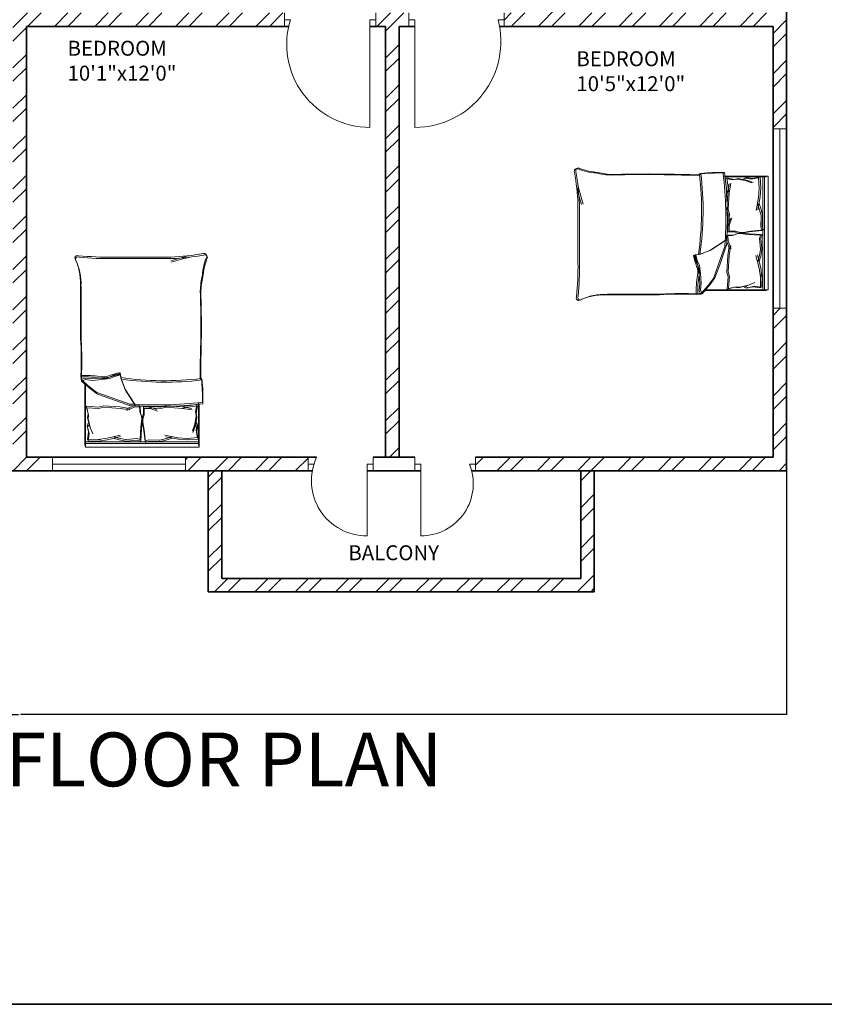
# Model space of a CAD drawing. Units: inches. Extents: x 1944 to 3454, y 1352 to 3055.
# Tile 3 of 17: x 2314 to 2582, y 1352 to 1681. Entities that reach past the tile are written whole.
import ezdxf

# ---------------------------------------------------------------- set-up
doc = ezdxf.new("R2010")
doc.units = ezdxf.units.IN
for name, color, linetype, lineweight in [('A-ANNO-DIMS', 2, 'Continuous', 18), ('A-ANNO-TITL', 7, 'Continuous', 30), ('A-ANNO-TTLB', 7, 'Continuous', 35), ('A-AREA-IDEN', 7, 'Continuous', 18), ('A-DOOR', 3, 'Continuous', 20), ('A-FURN', 8, 'Continuous', 13), ('A-GLAZ', 4, 'Continuous', 18), ('A-WALL', 7, 'Continuous', 35), ('A-WALL-PATT', 252, 'Continuous', 13)]:
    doc.layers.add(name, color=color, linetype=linetype, lineweight=lineweight)
doc.styles.get("Standard").update_dxf_attribs({"font": 'arial.ttf'})
doc.dimstyles.get("Standard").update_dxf_attribs({"dimtxt": 0.18, "dimasz": 0.18, "dimexe": 0.18, "dimexo": 0.0625, "dimgap": 0.09, "dimtad": 0, "dimtih": 1, "dimtoh": 1, "dimdec": 4, "dimzin": 0, "dimdsep": 46, "dimtxsty": 'Standard', "dimcen": 0.09, "dimadec": 0, "dimazin": 0, "dimtfac": 1, "dimtdec": 4, "dimtofl": 0, "dimtmove": 0, "dimatfit": 3, "dimfxl": 1, "dimtolj": 1, "dimtzin": 0, "dimarcsym": 0})

# ---------------------------------------------------------------- blocks, each defined once
blk = doc.blocks.new('BED-WITH-PILLOWS-01')
for p, q in [((0, 40.75), (21.15, 40.75)), ((0, 40.75), (21.15, 40.75)), ((0, 2.76), (0, 40.75)), ((0.51, 40.93), (21.66, 40.93)), ((0.51, 40.93), (21.66, 40.93)), ((1.22, 2.76), (1.22, 40.75)), ((1.22, 2.76), (1.22, 40.75)), ((1.73, 2.94), (1.73, 40.93)), ((1.73, 2.94), (1.73, 40.93)), ((2.03, 39.83), (1.96, 35.54)), ((2.03, 39.83), (1.96, 35.54)), ((2.03, 39.83), (4.58, 39.53)), ((2.03, 39.83), (4.58, 39.53)), ((2.54, 40.01), (2.46, 35.72)), ((2.54, 40.01), (2.46, 35.72)), ((2.54, 40.01), (5.09, 39.71)), ((2.54, 40.01), (5.09, 39.71)), ((4.58, 39.53), (6.63, 40.01)), ((4.58, 39.53), (6.63, 40.01)), ((5.09, 39.71), (7.14, 40.19)), ((5.09, 39.71), (7.14, 40.19)), ((9.4, 39.83), (6.56, 39.2)), ((9.4, 39.83), (6.56, 39.2)), ((6.63, 40.01), (7.46, 39.6)), ((6.63, 40.01), (7.46, 39.6)), ((9.91, 40.01), (7.07, 39.38)), ((9.91, 40.01), (7.07, 39.38)), ((7.14, 40.19), (7.97, 39.78)), ((7.14, 40.19), (7.97, 39.78)), ((10.68, 39.68), (9.4, 39.83)), ((10.68, 39.68), (9.4, 39.83)), ((11.19, 39.86), (9.91, 40.01)), ((11.19, 39.86), (9.91, 40.01)), ((13.17, 40.3), (10.68, 39.68)), ((13.17, 40.3), (10.68, 39.68)), ((13.68, 40.48), (11.19, 39.86)), ((13.68, 40.48), (11.19, 39.86)), ((12.85, 36.22), (13.17, 40.3)), ((12.85, 36.22), (13.17, 40.3)), ((13.36, 36.4), (13.68, 40.48)), ((13.36, 36.4), (13.68, 40.48)), ((22.05, 42.02), (19.47, 39.08)), ((22.05, 42.02), (19.47, 39.08)), ((22.56, 42.21), (19.98, 39.26)), ((22.56, 42.21), (19.98, 39.26)), ((23.44, 42.09), (22.05, 42.02, 3.08)), ((23.44, 42.09), (22.05, 42.02, 3.08)), ((22.55, 40.8), (22.05, 42.02)), ((22.55, 40.8), (22.05, 42.02)), ((22.3, 38.34), (22.55, 40.8)), ((22.3, 38.34), (22.55, 40.8)), ((23.95, 42.27), (22.56, 42.21, 3.08)), ((23.95, 42.27), (22.56, 42.21, 3.08)), ((23.05, 40.98), (22.56, 42.21)), ((23.05, 40.98), (22.56, 42.21)), ((22.81, 38.52), (23.05, 40.98)), ((22.81, 38.52), (23.05, 40.98)), ((1.96, 35.54), (2.02, 36.34)), ((1.96, 35.54), (2.02, 36.34)), ((2.02, 36.34), (2.44, 33.32)), ((2.02, 36.34), (2.44, 33.32)), ((2.46, 35.72), (2.53, 36.52)), ((2.46, 35.72), (2.53, 36.52)), ((2.53, 36.52), (2.95, 33.5)), ((2.53, 36.52), (2.95, 33.5)), ((6.56, 39.2), (4.43, 38.26)), ((6.56, 39.2), (4.43, 38.26)), ((7.07, 39.38), (4.94, 38.44)), ((7.07, 39.38), (4.94, 38.44)), ((13.3, 34.66), (12.85, 36.22)), ((13.3, 34.66), (12.85, 36.22)), ((13.8, 34.84), (13.36, 36.4)), ((13.8, 34.84), (13.36, 36.4)), ((17.75, 36.74), (16.15, 32.31)), ((17.75, 36.74), (16.15, 32.31)), ((18.26, 36.92), (16.66, 32.49)), ((18.26, 36.92), (16.66, 32.49)), ((19.47, 39.08), (17.75, 36.74)), ((19.47, 39.08), (17.75, 36.74)), ((19.98, 39.26), (18.26, 36.92)), ((19.98, 39.26), (18.26, 36.92)), ((22.55, 35.26), (22.3, 38.34)), ((22.55, 35.26), (22.3, 38.34)), ((23.05, 35.44), (22.81, 38.52)), ((23.05, 35.44), (22.81, 38.52)), ((2.44, 33.32), (3.51, 29.01)), ((2.44, 33.32), (3.51, 29.01)), ((2.95, 33.5), (4.02, 29.19)), ((2.95, 33.5), (4.02, 29.19)), ((12.95, 29.09), (13.3, 34.66)), ((12.95, 29.09), (13.3, 34.66)), ((13.46, 29.27), (13.8, 34.84)), ((13.46, 29.27), (13.8, 34.84)), ((22.92, 32.55), (22.55, 35.26)), ((22.92, 32.55), (22.55, 35.26)), ((23.42, 32.74), (23.05, 35.44)), ((23.42, 32.74), (23.05, 35.44)), ((2.92, 31.16), (2.45, 29.52)), ((2.92, 31.16), (2.45, 29.52)), ((2.95, 29.7), (2.52, 27.37)), ((2.95, 29.7), (2.52, 27.37)), ((3.43, 31.34), (2.95, 29.7)), ((3.43, 31.34), (2.95, 29.7)), ((16.15, 32.31), (13.82, 25.68)), ((16.15, 32.31), (13.82, 25.68)), ((16.66, 32.49), (14.33, 25.86)), ((16.66, 32.49), (14.33, 25.86)), ((23.65, 30.95), (22.92, 32.55)), ((23.65, 30.95), (22.92, 32.55)), ((24.16, 31.13), (23.42, 32.74)), ((24.16, 31.13), (23.42, 32.74)), ((24.15, 28.98), (23.65, 30.95)), ((24.15, 28.98), (23.65, 30.95)), ((24.65, 29.17), (24.16, 31.13)), ((24.65, 29.16), (24.16, 31.13)), ((62.99, 11.97), (62.99, 31.54)), ((62.99, 11.97), (62.99, 31.54)), ((63.5, 12.16), (63.5, 31.72)), ((63.5, 12.15), (63.5, 31.72)), ((2.45, 29.52), (2.02, 27.19)), ((2.45, 29.52), (2.02, 27.19)), ((2.02, 27.19), (2.03, 26.93)), ((2.02, 27.19), (2.03, 26.93)), ((2.03, 26.93), (2.37, 23.41)), ((2.03, 26.93), (2.37, 23.41)), ((2.52, 27.37), (2.54, 27.12)), ((2.52, 27.37), (2.54, 27.11)), ((2.54, 27.12), (2.88, 23.6)), ((2.54, 27.11), (2.88, 23.6)), ((13.31, 24.44), (12.28, 26.88)), ((13.31, 24.44), (12.28, 26.88)), ((12.42, 25.88), (12.95, 29.09)), ((12.42, 25.88), (12.95, 29.09)), ((13.81, 24.62), (12.79, 27.07)), ((13.81, 24.62), (12.79, 27.06)), ((12.93, 26.07), (13.46, 29.27)), ((12.93, 26.07), (13.46, 29.27)), ((13.82, 24.05), (18.98, 27.38)), ((13.82, 24.05), (18.98, 27.38)), ((14.33, 24.23), (19.49, 27.56)), ((14.33, 24.23), (19.49, 27.56)), ((18.98, 27.38), (22.55, 28.74)), ((18.98, 27.38), (22.55, 28.74)), ((19.49, 27.56), (23.05, 28.92)), ((19.49, 27.56), (23.05, 28.92)), ((22.55, 28.74), (24.15, 28.98)), ((22.55, 28.74), (24.15, 28.98)), ((23.05, 28.92), (24.65, 29.17)), ((23.05, 28.92), (24.65, 29.16)), ((2.37, 23.41), (1.98, 22.24)), ((2.37, 23.41), (1.98, 22.24)), ((2.88, 23.6), (2.49, 22.42)), ((2.88, 23.6), (2.49, 22.42)), ((13.43, 22.49), (13.31, 24.44)), ((13.43, 22.49), (13.31, 24.44)), ((13.94, 22.67), (13.81, 24.62)), ((13.94, 22.67), (13.81, 24.62)), ((1.49, 20.65), (5.74, 21.11)), ((1.49, 20.65), (5.74, 21.11)), ((1.95, 19.5), (1.49, 20.65)), ((1.95, 19.5), (1.49, 20.65)), ((1.98, 22.24), (6.25, 22.04)), ((1.98, 22.24), (6.25, 22.04)), ((1.99, 20.83), (6.25, 21.29)), ((1.99, 20.83), (6.25, 21.29)), ((2.45, 19.69), (1.99, 20.83)), ((2.45, 19.69), (1.99, 20.83)), ((2.49, 22.42), (6.76, 22.23)), ((2.49, 22.42), (6.76, 22.23)), ((5.74, 21.11), (8.27, 21.57)), ((5.74, 21.11), (8.27, 21.57)), ((6.25, 22.04), (8.81, 21.74)), ((6.25, 22.04), (8.81, 21.74)), ((6.25, 21.29), (8.78, 21.75)), ((6.25, 21.29), (8.78, 21.75)), ((6.76, 22.23), (9.31, 21.93)), ((6.76, 22.23), (9.31, 21.93)), ((8.27, 21.57), (9.3, 21.57)), ((8.27, 21.57), (9.3, 21.57)), ((8.78, 21.75), (9.81, 21.75)), ((8.78, 21.75), (9.81, 21.75)), ((8.81, 21.74), (9.84, 21.81)), ((8.81, 21.74), (9.84, 21.81)), ((9.3, 21.57), (10.8, 21.11)), ((9.3, 21.57), (10.8, 21.11)), ((9.31, 21.93), (10.35, 21.99)), ((9.31, 21.93), (10.35, 21.99)), ((9.81, 21.75), (11.3, 21.29)), ((9.81, 21.75), (11.3, 21.29)), ((9.84, 21.81), (11.3, 22.36)), ((9.84, 21.81), (11.3, 22.36)), ((10.35, 21.99), (11.81, 22.54)), ((10.35, 21.99), (11.81, 22.54)), ((10.8, 21.11), (12.93, 21.11)), ((10.8, 21.11), (12.93, 21.11)), ((11.3, 22.36), (13.43, 22.49)), ((11.3, 22.36), (13.43, 22.49)), ((11.3, 21.29), (13.44, 21.29)), ((11.3, 21.29), (13.44, 21.29)), ((11.81, 22.54), (13.94, 22.67)), ((11.81, 22.54), (13.94, 22.67)), ((12.93, 21.11), (12.93, 19.16)), ((12.93, 21.11), (12.93, 19.16)), ((13.44, 21.29), (13.44, 19.34)), ((13.44, 21.29), (13.44, 19.34)), ((1.83, 15.97), (1.95, 19.5)), ((1.83, 15.97), (1.95, 19.5)), ((2.34, 16.15), (2.45, 19.69)), ((2.34, 16.15), (2.45, 19.69)), ((12.93, 19.16), (12.06, 16.66)), ((12.93, 19.16), (12.06, 16.66)), ((13.44, 19.34), (12.57, 16.84)), ((13.44, 19.34), (12.57, 16.84)), ((12.85, 15.41), (13.17, 19.49)), ((12.85, 15.41), (13.17, 19.49)), ((13.36, 15.59), (13.68, 19.67)), ((13.36, 15.59), (13.68, 19.67)), ((1.83, 15.71), (1.83, 15.97)), ((1.83, 15.71), (1.83, 15.97)), ((2.41, 13.42), (1.83, 15.71)), ((2.41, 13.42), (1.83, 15.71)), ((2.34, 15.9), (2.34, 16.15)), ((2.34, 15.9), (2.34, 16.15)), ((2.91, 13.6), (2.34, 15.9)), ((2.91, 13.6), (2.34, 15.9)), ((2.98, 11.81), (2.41, 13.42)), ((2.98, 11.81), (2.41, 13.42)), ((2.64, 9.62), (3.44, 13.99)), ((2.64, 9.62), (3.44, 13.99)), ((3.49, 11.99), (2.91, 13.6)), ((3.49, 11.99), (2.91, 13.6)), ((3.14, 9.81), (3.95, 14.17)), ((3.14, 9.81), (3.95, 14.17)), ((13.3, 13.85), (12.85, 15.41)), ((13.3, 13.85), (12.85, 15.41)), ((12.95, 8.28), (13.3, 13.85)), ((12.95, 8.28), (13.3, 13.85)), ((13.8, 14.03), (13.36, 15.59)), ((13.8, 14.03), (13.36, 15.59)), ((13.46, 8.46), (13.8, 14.03)), ((13.46, 8.46), (13.8, 14.03)), ((2.39, 6.5), (2.41, 6.59)), ((2.39, 6.5), (2.41, 6.59)), ((2.41, 6.59), (2.64, 9.62)), ((2.41, 6.59), (2.64, 9.62)), ((2.9, 6.68), (2.91, 6.77)), ((2.9, 6.68), (2.91, 6.77)), ((3.16, 3.28), (2.9, 6.68)), ((3.16, 3.28), (2.9, 6.68)), ((2.91, 6.77), (3.14, 9.81)), ((2.91, 6.77), (3.14, 9.81)), ((12.42, 5.07), (12.95, 8.28)), ((12.42, 5.07), (12.95, 8.28)), ((12.93, 5.25), (13.46, 8.46)), ((12.93, 5.25), (13.46, 8.46)), ((12.95, 8.28), (13.21, 7.38)), ((12.95, 8.28), (13.21, 7.38)), ((13.21, 7.38), (13.78, 3.33)), ((13.21, 7.38), (13.78, 3.33)), ((13.46, 8.46), (13.72, 7.56)), ((13.46, 8.46), (13.72, 7.56)), ((13.72, 7.56), (14.29, 3.51)), ((13.72, 7.56), (14.29, 3.51)), ((2.65, 3.1), (2.39, 6.5)), ((2.65, 3.1), (2.39, 6.5)), ((2.64, 3.1), (5.16, 3.56)), ((2.64, 3.1), (5.16, 3.56)), ((3.14, 3.28), (5.67, 3.74)), ((3.14, 3.28), (5.67, 3.74)), ((7.12, 4.02), (4.93, 4.82)), ((7.12, 4.01), (4.93, 4.82)), ((5.16, 3.56), (7.23, 3.21)), ((5.16, 3.56), (7.23, 3.21)), ((7.63, 4.2), (5.44, 5)), ((7.63, 4.2), (5.44, 5)), ((5.67, 3.74), (7.74, 3.39)), ((5.67, 3.74), (7.74, 3.39)), ((9.99, 3.56), (7.12, 4.02)), ((9.99, 3.56), (7.12, 4.01)), ((7.23, 3.21), (8.04, 3.67)), ((7.23, 3.21), (8.04, 3.67)), ((10.5, 3.74), (7.63, 4.2)), ((10.5, 3.74), (7.63, 4.2)), ((7.74, 3.39), (8.55, 3.85)), ((7.74, 3.39), (8.55, 3.85)), ((11.26, 3.79), (9.99, 3.56)), ((11.26, 3.79), (9.99, 3.56)), ((11.76, 3.97), (10.5, 3.74)), ((11.76, 3.97), (10.5, 3.74)), ((13.78, 3.33), (11.26, 3.79)), ((13.78, 3.33), (11.26, 3.79)), ((14.29, 3.51), (11.76, 3.97)), ((14.29, 3.51), (11.76, 3.97)), ((14.4, 2.76), (0, 2.76)), ((14.4, 2.76), (0, 2.76)), ((14.9, 2.94), (0.51, 2.94)), ((14.9, 2.94), (0.51, 2.94))]:
    blk.add_line(p, q)
for centre, radius, start, end in [((54.58, 60.54), 18.33, 267.4714, 296.4681), ((54.58, 60.54), 18.33, 267.4714, 296.4681), ((55.09, 60.72), 18.33, 267.4714, 296.4681), ((55.09, 60.72), 18.33, 267.4714, 296.4681), ((62.69, 43.25), 0.876, 332.6588, 86.02), ((62.69, 43.25), 0.876, 332.6588, 86.02), ((168.74, 32.71), 105.75, 174.4998, 180.6351), ((168.74, 32.71), 105.75, 174.4998, 180.6351), ((63.2, 43.43), 0.876, 332.6588, 86.02), ((63.2, 43.43), 0.876, 332.6588, 86.02), ((169.24, 32.89), 105.75, 174.4998, 180.6351), ((169.24, 32.89), 105.75, 174.4998, 180.6351), ((-5.29, 40.8), 28.76, 349.8763, 2.5657), ((-5.29, 40.8), 28.76, 349.8763, 2.5657), ((28.87, 144.88), 102.94, 266.9791, 273.8365), ((28.87, 144.88), 102.94, 266.9791, 273.8365), ((-4.78, 40.98), 28.76, 349.8763, 2.5657), ((-4.78, 40.98), 28.76, 349.8763, 2.5657), ((29.37, 145.06), 102.94, 266.9791, 273.8365), ((29.37, 145.06), 102.94, 266.9791, 273.8365), ((53.91, -3583.94), 3626.16, 90.00217, 90.28689), ((53.91, -3583.94), 3626.16, 90.00217, 90.28689), ((54.42, -3583.76), 3626.16, 90.00217, 90.28689), ((54.42, -3583.76), 3626.16, 90.00217, 90.28689), ((27.87, 34.77), 4.95, 168.6608, 203.7384), ((27.87, 34.77), 4.95, 168.6608, 203.7384), ((28.38, 34.95), 4.95, 168.6608, 203.7384), ((28.38, 34.95), 4.95, 168.6608, 203.7384), ((1.69, 24.95), 23.57, 10.6617, 19.8806), ((1.69, 24.94), 23.57, 10.6617, 19.8806), ((1.18, 24.76), 23.57, 10.6617, 19.8806), ((1.18, 24.76), 23.57, 10.6617, 19.8806), ((124.25, 14.11), 102.56, 171.7845, 186.9006), ((124.25, 14.11), 102.56, 171.7845, 186.9006), ((124.76, 14.3), 102.56, 171.7845, 186.9006), ((124.76, 14.3), 102.56, 171.7845, 186.9006), ((24.2, 29.12), 0.147, 250.2464, 1.1377), ((24.2, 29.12), 0.147, 250.2464, 1.1377), ((24.7, 29.3), 0.147, 250.2464, 1.1377), ((24.7, 29.3), 0.147, 250.2464, 1.1377), ((144.71, 16.98), 131.13, 176.0865, 186.7821), ((144.71, 16.98), 131.13, 176.0865, 186.7821), ((145.22, 17.16), 131.13, 176.0865, 186.7821), ((145.22, 17.16), 131.13, 176.0865, 186.7821), ((-18.85, -13.69), 84.62, 13.3832, 17.7053), ((-18.85, -13.69), 84.62, 13.3832, 17.7053), ((-18.34, -13.51), 84.62, 13.3832, 17.7053), ((-18.34, -13.51), 84.62, 13.3832, 17.7053), ((159.64, 17.03), 96.78, 182.9958, 189.4091), ((159.64, 17.03), 96.78, 182.9958, 189.4091), ((160.15, 17.21), 96.78, 182.9958, 189.4091), ((160.15, 17.21), 96.78, 182.9958, 189.4091), ((15.97, 67.69), 66.22, 268.7218, 275.604), ((15.97, 67.69), 66.22, 268.7218, 275.604), ((16.48, 67.88), 66.22, 268.7218, 275.604), ((16.48, 67.88), 66.22, 268.7218, 275.604), ((24.78, -132.99), 135.22, 88.4762, 91.0082), ((24.78, -132.99), 135.22, 88.4762, 91.0082), ((25.29, -132.81), 135.22, 88.4762, 91.0082), ((25.29, -132.81), 135.22, 88.4762, 91.0082), ((40.23, 385.38), 383.38, 268.2277, 271.7185), ((40.23, 385.38), 383.38, 268.2277, 271.7185), ((40.74, 385.56), 383.38, 268.2277, 271.7185), ((40.74, 385.56), 383.38, 268.2277, 271.7185), ((51.28, -21.38), 23.56, 76.0648, 88.9113), ((51.28, -21.38), 23.56, 76.0648, 88.9113), ((51.79, -21.2), 23.56, 76.0648, 88.9113), ((51.79, -21.2), 23.56, 76.0648, 88.9113), ((55.86, -17.22), 18.73, 67.9751, 86.652), ((55.86, -17.22), 18.73, 67.9751, 86.652), ((56.37, -17.04), 18.73, 67.9751, 86.652), ((56.37, -17.04), 18.73, 67.9751, 86.652), ((63.37, 0.86), 0.866, 236.1736, 23.4781), ((63.37, 0.86), 0.866, 236.1736, 23.4781), ((63.87, 1.05), 0.866, 236.1736, 23.4781), ((63.87, 1.05), 0.866, 236.1736, 23.4781)]:
    blk.add_arc(centre, radius, start, end)
blk = doc.blocks.new('DOOR-SWING-36IN-05')
for p, q in [((0, 33.75), (0, 38.25)), ((0, 38.25), (0, 36)), ((31.76, 33.75), (31.76, 38.25)), ((31.76, 38.25), (31.76, 36)), ((0, 36), (0, 36)), ((0, 36), (2, 36)), ((2, 36), (2, 0)), ((31.76, 36), (29.76, 36))]:
    blk.add_line(p, q)
blk.add_arc((2, 28.7), 28.7, 270, 14.7288)
blk = doc.blocks.new('DOOR-SWING-36IN-06')
for p, q in [((0, 33.75), (0, 38.25)), ((0, 38.25), (0, 36)), ((30.6, 33.75), (30.6, 38.25)), ((30.6, 38.25), (30.6, 36)), ((0, 36), (2, 36)), ((30.6, 36), (28.6, 36)), ((28.6, 36), (28.6, 0))]:
    blk.add_line(p, q)
blk.add_arc((28.6, 27.83), 27.83, 162.9212, 270)
blk = doc.blocks.new('DOOR-SWING-24IN-11')
for p, q in [((0, 21.75), (0, 26.25)), ((0, 26.25), (0, 24)), ((0, 24), (2, 24)), ((21.74, 24), (19.74, 24)), ((19.74, 24), (19.74, 0)), ((21.74, 26.25), (21.74, 21.75)), ((21.74, 21.75), (21.74, 24))]:
    blk.add_line(p, q)
blk.add_arc((19.54, 18.41), 18.41, 154.7737, 270.6503)
blk = doc.blocks.new('DOOR-SWING-24IN-12')
for p, q in [((0, 26.25), (0, 21.75)), ((0, 21.75), (0, 24)), ((0, 24), (2, 24)), ((2, 24), (2, 0)), ((20.24, 24), (18.24, 24)), ((20.24, 26.25), (20.24, 21.75)), ((20.24, 21.75), (20.24, 24))]:
    blk.add_line(p, q)
blk.add_arc((2.03, 17.47), 17.47, 269.8982, 21.9448)
blk = doc.blocks.new('WINDOW-PLAN-60.00IN-01')
for p, q in [((0, 60), (4.5, 60)), ((4.5, 60), (2.25, 60)), ((2.25, 60), (2.25, 0)), ((4.5, 0), (0, 0)), ((2.25, 0), (4.5, 0))]:
    blk.add_line(p, q)
blk = doc.blocks.new('WINDOW-PLAN-44.51IN-01')
for p, q in [((0, 4.5), (0, 0)), ((44.51, 2.25), (44.51, 4.5)), ((44.51, 4.5), (44.51, 0)), ((0, 0), (0, 2.25)), ((0, 2.25), (44.51, 2.25))]:
    blk.add_line(p, q)
blk = doc.blocks.new('*D184')
at = {"layer": 'A-ANNO-DIMS', "color": 0, "lineweight": -2, "transparency": 16777216}
for p, q in [((2057.32, 1530.03), (2057.32, 1448.47)), ((2569.82, 1530.03), (2569.82, 1448.47)), ((2057.5, 1448.65), (2313.18, 1448.65)), ((2569.64, 1448.65), (2313.97, 1448.65))]:
    blk.add_line(p, q, dxfattribs=at)
at = {"layer": 'A-ANNO-DIMS', "color": 0, "transparency": 16777216}
for points in [[(2057.5, 1448.68), (2057.5, 1448.62), (2057.32, 1448.65)], [(2569.64, 1448.68), (2569.64, 1448.62), (2569.82, 1448.65)]]:
    blk.add_solid(points, dxfattribs=at)
at = {"layer": 'Defpoints', "color": 0, "transparency": 16777216}
for p in [(2057.32, 1530.1), (2569.82, 1530.1), (2569.82, 1448.65)]:
    blk.add_point(p, dxfattribs=at)
at = {"layer": 'A-ANNO-DIMS', "color": 0, "transparency": 16777216, "insert": (2313.57, 1448.65), "char_height": 0.18, "attachment_point": 5}
blk.add_mtext('\\A1;512.5', dxfattribs=at)

msp = doc.modelspace()

# ---------------------------------------------------------------- hatches: boundary and pattern name
at = {"layer": 'A-WALL-PATT'}
h = msp.add_hatch(dxfattribs=at)
h.set_pattern_fill('ANSI32', color=256)
h.paths.add_polyline_path([(2061.822, 2177.596), (2158.181, 2177.596), (2158.181, 2179.846), (2158.181, 2182.096), (2057.322, 2182.096), (2057.322, 2123.452), (2061.822, 2123.452)])
h.paths.add_polyline_path([(2258.993, 2179.846), (2258.993, 2182.096), (2218.838, 2182.096), (2218.838, 2177.596), (2258.993, 2177.596)])
h.paths.add_polyline_path([(2315.822, 2177.596), (2322.722, 2177.596), (2322.722, 2182.096), (2303.186, 2182.096), (2303.186, 2177.596), (2311.322, 2177.596), (2311.322, 2033.596), (2231.355, 2033.596), (2231.355, 2029.096), (2311.322, 2029.096), (2311.322, 1904.596), (2307.941, 1904.596), (2307.941, 1900.096), (2319.277, 1900.096), (2319.277, 1902.346), (2319.277, 1904.596), (2315.822, 1904.596), (2315.822, 2029.096), (2394.855, 2029.096), (2394.855, 2033.596), (2315.822, 2033.596)])
h.paths.add_polyline_path([(2407.334, 2182.096), (2366.1, 2182.096), (2366.1, 2177.596), (2407.334, 2177.596), (2407.334, 2179.846)])
h.paths.add_polyline_path([(2440.322, 2177.596), (2443.866, 2177.596), (2443.866, 2182.096), (2431.827, 2182.096), (2431.827, 2179.846), (2431.827, 2177.596), (2435.822, 2177.596), (2435.822, 2033.596), (2430.464, 2033.596), (2430.464, 2029.096), (2445.372, 2029.096), (2445.372, 2031.346), (2445.372, 2033.596), (2440.322, 2033.596)])
h.paths.add_polyline_path([(2569.822, 2182.096), (2466.481, 2182.096), (2466.481, 2177.596), (2565.322, 2177.596), (2565.322, 2123.452), (2569.822, 2123.452)])
h.paths.add_polyline_path([(2569.822, 2063.452), (2567.572, 2063.452), (2565.322, 2063.452), (2565.322, 2033.596), (2478.08, 2033.596), (2476.822, 2033.596), (2476.822, 2028.698), (2476.822, 2020.069), (2481.322, 2020.069), (2481.322, 2029.096), (2565.322, 2029.096), (2565.322, 2014.5), (2569.822, 2014.5)])
h.paths.add_polyline_path([(2569.822, 1978.5), (2565.322, 1978.5), (2565.322, 1957.096), (2481.322, 1957.096), (2481.322, 1990.369), (2476.822, 1990.369), (2476.822, 1957.096), (2476.822, 1952.596), (2476.822, 1947.471), (2481.322, 1947.471), (2481.322, 1952.596), (2565.322, 1952.596), (2565.322, 1943.2), (2569.822, 1943.2)])
h.paths.add_polyline_path([(2569.822, 1919.2), (2565.322, 1919.2), (2565.322, 1904.596), (2481.322, 1904.596), (2481.322, 1928.596), (2476.822, 1928.596), (2476.822, 1904.596), (2350.518, 1904.596), (2350.518, 1900.096), (2476.822, 1900.096), (2565.322, 1900.096), (2565.322, 1895.596), (2565.322, 1887.047), (2569.822, 1887.047)])
h.paths.add_polyline_path([(2280.492, 1904.596), (2150.322, 1904.596), (2150.322, 1926.68), (2148.072, 1926.68), (2145.822, 1926.68), (2145.822, 1904.596), (2061.822, 1904.596), (2061.822, 1914.977), (2059.572, 1914.977), (2057.322, 1914.977), (2057.322, 1887.362), (2061.822, 1887.362), (2061.822, 1900.096), (2150.322, 1900.096), (2280.492, 1900.096), (2280.492, 1902.346)])
h.paths.add_polyline_path([(2150.322, 1957.096), (2150.322, 1986.22), (2145.822, 1986.22), (2145.822, 1957.096), (2061.822, 1957.096), (2061.822, 1975.678), (2057.322, 1975.678), (2057.322, 1938.977), (2061.822, 1938.977), (2061.822, 1952.596), (2145.822, 1952.596), (2145.822, 1947.985), (2150.322, 1947.985), (2150.322, 1952.596)])
h.paths.add_polyline_path([(2061.822, 2063.452), (2057.322, 2063.452), (2057.322, 2011.678), (2061.822, 2011.678), (2061.822, 2029.096), (2145.288, 2029.096), (2145.822, 2029.096), (2145.822, 2019.118), (2150.322, 2019.118), (2150.322, 2029.096), (2150.322, 2033.596), (2147.022, 2033.596), (2061.822, 2033.596)])
h.paths.add_polyline_path([(2061.822, 1835.596), (2133.822, 1835.596), (2133.822, 1794.415), (2138.322, 1794.415), (2138.322, 1835.596), (2231.726, 1835.596), (2231.726, 1840.096), (2061.822, 1840.096), (2061.822, 1851.362), (2057.322, 1851.362), (2057.322, 1810.528), (2061.822, 1810.528)])
h.paths.add_polyline_path([(2061.822, 1774.528), (2059.572, 1774.528), (2057.322, 1774.528), (2057.322, 1723.746), (2061.822, 1723.746), (2061.822, 1735.096), (2133.822, 1735.096), (2133.822, 1731.415), (2138.322, 1731.415), (2138.322, 1759.737), (2133.822, 1759.737), (2133.822, 1739.596), (2061.822, 1739.596)])
h.paths.add_polyline_path([(2061.822, 1678.596), (2147.597, 1678.596), (2147.597, 1680.846), (2147.597, 1683.096), (2138.322, 1683.096), (2138.322, 1710.66), (2136.072, 1710.66), (2133.822, 1710.66), (2133.822, 1683.096), (2061.822, 1683.096), (2061.822, 1699.746), (2057.322, 1699.746), (2057.322, 1645.751), (2061.822, 1645.751)])
h.paths.add_polyline_path([(2061.822, 1585.751), (2057.322, 1585.751), (2057.322, 1530.096), (2158.703, 1530.096), (2158.703, 1534.596), (2061.822, 1534.596)])
h.paths.add_polyline_path([(2191.322, 1678.596), (2195.889, 1678.596), (2195.889, 1683.096), (2181.763, 1683.096), (2181.763, 1680.846), (2181.763, 1678.596), (2186.822, 1678.596), (2186.822, 1534.596), (2181.354, 1534.596), (2181.354, 1530.096), (2196.54, 1530.096), (2196.54, 1532.346), (2196.54, 1534.596), (2191.322, 1534.596)])
h.paths.add_polyline_path([(2315.822, 1678.596), (2402.014, 1678.596), (2402.014, 1683.096), (2355.822, 1683.096), (2355.822, 1835.596), (2360.838, 1835.596), (2360.838, 1840.096), (2351.322, 1840.096), (2351.322, 1683.096), (2273.322, 1683.096), (2273.322, 1840.096), (2263.134, 1840.096), (2263.134, 1837.846), (2263.134, 1835.596), (2268.822, 1835.596), (2268.822, 1683.096), (2227.793, 1683.096), (2227.793, 1678.596), (2311.322, 1678.596), (2311.322, 1534.596), (2302.384, 1534.596), (2302.384, 1530.096), (2324.521, 1530.096), (2324.521, 1532.346), (2324.521, 1534.596), (2315.822, 1534.596)])
h.paths.add_polyline_path([(2440.322, 1678.596), (2443.656, 1678.596), (2443.656, 1683.096), (2432.614, 1683.096), (2432.614, 1680.846), (2432.614, 1678.596), (2435.822, 1678.596), (2435.822, 1534.596), (2440.322, 1534.596)])
h.paths.add_polyline_path([(2409.913, 1534.596), (2369.033, 1534.596), (2369.033, 1530.096), (2409.913, 1530.096)])
h.paths.add_polyline_path([(2259.529, 1532.346), (2259.529, 1534.596), (2218.889, 1534.596), (2218.889, 1532.346), (2218.889, 1530.096), (2259.529, 1530.096)])
h.paths.add_polyline_path([(2569.822, 1584.389), (2567.572, 1584.389), (2565.322, 1584.389), (2565.322, 1534.596), (2465.892, 1534.596), (2465.892, 1530.096), (2569.822, 1530.096)])
h.paths.add_polyline_path([(2505.567, 1530.096), (2501.067, 1530.096), (2501.067, 1494.096), (2381.067, 1494.096), (2381.067, 1530.096), (2376.567, 1530.096), (2376.567, 1489.596), (2381.067, 1489.596), (2505.567, 1489.596), (2505.567, 1494.096)])
h.paths.add_polyline_path([(2127.673, 1530.096), (2123.173, 1530.096), (2123.173, 1489.596), (2127.673, 1489.596), (2252.173, 1489.596), (2252.173, 1494.096), (2252.173, 1530.096), (2247.673, 1530.096), (2247.673, 1494.096), (2127.673, 1494.096)])
h.paths.add_polyline_path([(2251.167, 2222.596), (2126.667, 2222.596), (2122.167, 2222.596), (2122.167, 2182.096), (2126.667, 2182.096), (2126.667, 2218.096), (2210.667, 2218.096), (2234.667, 2218.096), (2246.667, 2218.096), (2246.667, 2182.096), (2251.167, 2182.096), (2251.167, 2218.096)])
h.paths.add_polyline_path([(2501.916, 2222.596), (2497.416, 2222.596), (2372.916, 2222.596), (2372.916, 2218.096), (2372.916, 2182.096), (2377.416, 2182.096), (2377.416, 2218.096), (2497.416, 2218.096), (2497.416, 2182.096), (2501.916, 2182.096)])
h.paths.add_polyline_path([(2569.822, 1700.442), (2565.322, 1700.442), (2565.322, 1683.096), (2493.322, 1683.096), (2493.322, 1709.096), (2488.822, 1709.096), (2488.822, 1683.096), (2475.416, 1683.096), (2475.416, 1680.846), (2475.416, 1678.596), (2488.822, 1678.596), (2565.322, 1678.596), (2565.322, 1644.389), (2569.822, 1644.389)])
h.paths.add_polyline_path([(2569.822, 1773.506), (2565.322, 1773.506), (2565.322, 1739.596), (2493.322, 1739.596), (2493.322, 1754.002), (2488.822, 1754.002), (2488.822, 1729.846), (2491.072, 1729.846), (2493.322, 1729.846), (2493.322, 1735.096), (2565.322, 1735.096), (2565.322, 1724.442), (2569.822, 1724.442)])
h.paths.add_polyline_path([(2569.822, 1851.047), (2567.572, 1851.047), (2565.322, 1851.047), (2565.322, 1840.096), (2395.039, 1840.096), (2395.039, 1837.846), (2395.039, 1835.596), (2488.822, 1835.596), (2488.822, 1798.423), (2493.322, 1798.423), (2493.322, 1835.596), (2565.322, 1835.596), (2565.322, 1809.506), (2569.822, 1809.506)])
h.paths.add_polyline_path([(2347.275, 1955.576), (2414.024, 1955.576), (2414.024, 1974.234), (2347.275, 1974.234)], flags=9)
h.paths.add_polyline_path([(2509.756, 1990.497), (2542.915, 1990.497), (2542.915, 2009.154), (2509.756, 2009.154)], flags=9)

# ---------------------------------------------------------------- linework, layer by layer
at = {"layer": 'A-ANNO-TTLB'}
msp.add_lwpolyline([(1943.914, 3054.605), (3453.633, 3054.605), (3453.633, 1351.76), (1943.914, 1351.76)], close=True, dxfattribs=at)
at = {"layer": 'A-WALL'}
for p, q in [((2569.822, 2182.096), (2569.822, 1530.096)), ((2315.822, 1678.596), (2315.822, 1534.596)), ((2315.822, 1678.596), (2403.424, 1678.596)), ((2430.614, 1678.596), (2435.822, 1678.596)), ((2435.822, 1678.596), (2435.822, 1534.596)), ((2440.322, 1678.596), (2440.322, 1534.596)), ((2440.322, 1678.596), (2445.656, 1678.596)), ((2473.912, 1678.596), (2488.822, 1678.596)), ((2488.822, 1678.596), (2565.322, 1678.596)), ((2565.322, 1678.596), (2565.322, 1534.596)), ((2315.822, 1534.596), (2412.798, 1534.596)), ((2431.658, 1534.596), (2445.656, 1534.596)), ((2465.892, 1534.596), (2565.322, 1534.596)), ((2217.356, 1530.096), (2411.349, 1530.096)), ((2376.567, 1489.596), (2376.567, 1530.096)), ((2381.067, 1530.096), (2381.067, 1494.096)), ((2429.658, 1530.096), (2447.656, 1530.096)), ((2464.626, 1530.096), (2569.822, 1530.096)), ((2501.067, 1494.096), (2501.067, 1530.096)), ((2501.067, 1530.096), (2505.567, 1530.096)), ((2505.567, 1530.096), (2505.567, 1494.096)), ((2381.067, 1494.096), (2501.067, 1494.096)), ((2505.567, 1494.096), (2505.567, 1489.596)), ((2381.067, 1489.596), (2376.567, 1489.596)), ((2505.567, 1489.596), (2381.067, 1489.596))]:
    msp.add_line(p, q, dxfattribs=at)

# ---------------------------------------------------------------- block references
at = {"layer": 'A-DOOR'}
for name, p in [('DOOR-SWING-36IN-06', (2402.014, 1644.846)), ('DOOR-SWING-36IN-05', (2443.656, 1644.846)), ('DOOR-SWING-24IN-11', (2409.913, 1508.346)), ('DOOR-SWING-24IN-12', (2445.656, 1508.346))]:
    msp.add_blockref(name, p, dxfattribs=at)
at = {"layer": 'A-FURN'}
for p, rotation in [((2563.624, 1631.274), 180), ((2376.28, 1537.991), 90)]:
    msp.add_blockref('BED-WITH-PILLOWS-01', p, dxfattribs=dict(at, rotation=rotation))
at = {"layer": 'A-GLAZ'}
for name, p in [('WINDOW-PLAN-60.00IN-01', (2565.322, 1584.389)), ('WINDOW-PLAN-44.51IN-01', (2324.521, 1530.096))]:
    msp.add_blockref(name, p, dxfattribs=at)

# ---------------------------------------------------------------- texts
at = {"layer": 'A-ANNO-TITL', "insert": (2237.641, 1442.6), "char_height": 18, "attachment_point": 1}
msp.add_mtext_dynamic_manual_height_columns('FIRST FLOOR PLAN ', width=474.17053, gutter_width=12.5, heights=[0], dxfattribs=at)
at = {"layer": 'A-AREA-IDEN', "char_height": 5, "attachment_point": 1}
for s, width, insert in [('BEDROOM\\P10\'1"x12\'0"', 190.00606, (2329.563, 1673.806)), ('BEDROOM\\P10\'5"x12\'0"', 201.44708, (2499.585, 1670.294)), ('BALCONY', 118.50767, (2423.398, 1505.176))]:
    msp.add_mtext_dynamic_manual_height_columns(s, width=width, gutter_width=12.5, heights=[0], dxfattribs=dict(at, insert=insert))

# ---------------------------------------------------------------- dimensions: what is measured, and where the dimension line sits
at = {"layer": 'A-ANNO-DIMS'}
dim = msp.add_linear_dim(base=(2569.822, 1448.646), p1=(2057.322, 1530.096), p2=(2569.822, 1530.096), dimstyle='Standard', override={"dimdec": 1, "dimlfac": 1, "dimrnd": 0, "dimzin": 0, "dimdsep": 46, "dimlunit": 2}, dxfattribs=at)
dim.commit()
dim.dimension.update_dxf_attribs({"geometry": '*D184', "text_midpoint": (2313.572, 1448.646)})

doc.saveas('drawing.dxf')
